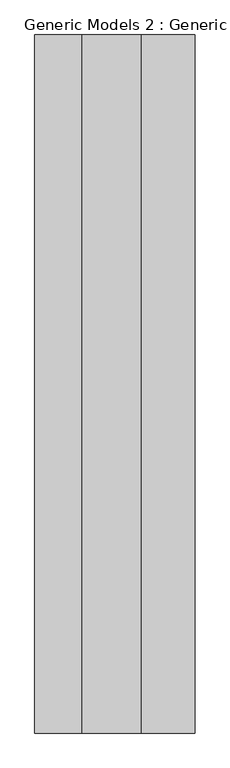
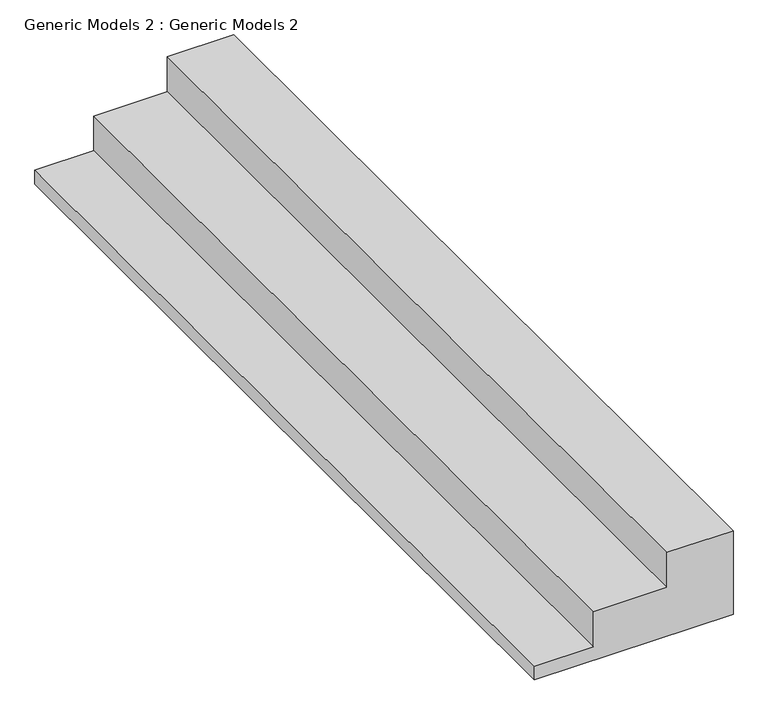
"""IFC4 building model written with IfcOpenShell, lengths in millimetres: proxy geometry, Generic Models 2 : Generic Models 2."""

from ifc_helpers import new_model, si_unit, frame, origin, place, context, project, spatial, polyline, outline, extrude, source, transform, mapped, element, save


def generic_models_2_generic_models_2_299d73bb(model_context):
    return source(origin(), model_context, "Body", "SweptSolid", [
        extrude(outline(polyline([(304.8, 23.3671209), (177.8, 23.3671209), (177.8, -230.6328791), (50.8, -230.6328791), (50.8, -433.8328791), (0.0, -433.8328791), (0.0, 251.9671209), (304.8, 251.9671209), (304.8, 23.3671209)])), frame((0.0, 5767.0223211, 0.0), z_axis=(0.0, 1.0, 0.0), x_axis=(0.0, 0.0, 1.0)), (0.0, 0.0, 1.0), 2984.5),
    ])


if __name__ == "__main__":
    model = new_model("IFC4")
    model_context = context("Model", 3, world=origin())
    ifc_project = project(units=[si_unit("LENGTHUNIT", "METRE", prefix="MILLI")], contexts=[model_context])
    site = spatial("IfcSite", under=ifc_project)
    building = spatial("IfcBuilding", under=site)
    placement = place(None, origin())
    generic_models_2_generic_models_2_shape = generic_models_2_generic_models_2_299d73bb(model_context)
    element("IfcBuildingElementProxy", 1, Name="Generic Models 2 : Generic Models 2", ObjectType="Generic Models 2 : Generic Models 2", at=placement, inside=building, context=model_context, shape_type="MappedRepresentation", body=[
        mapped(generic_models_2_generic_models_2_shape, transform((0.0, 0.0, 0.0), x_axis=(1.0, 0.0, 0.0), y_axis=(0.0, 1.0, 0.0), z_axis=(0.0, 0.0, 1.0))),
    ])
    save(model, "model.ifc")

# Revit data of these elements
# Element 1 (IfcBuildingElementProxy, "Generic Models 2 : Generic Models 2")
#   Materials on its faces: "Clad - White"
# Materials
#   "Clad - White": class "Wood", colour RGB 242 242 238, transparency 0, Cost = 0
